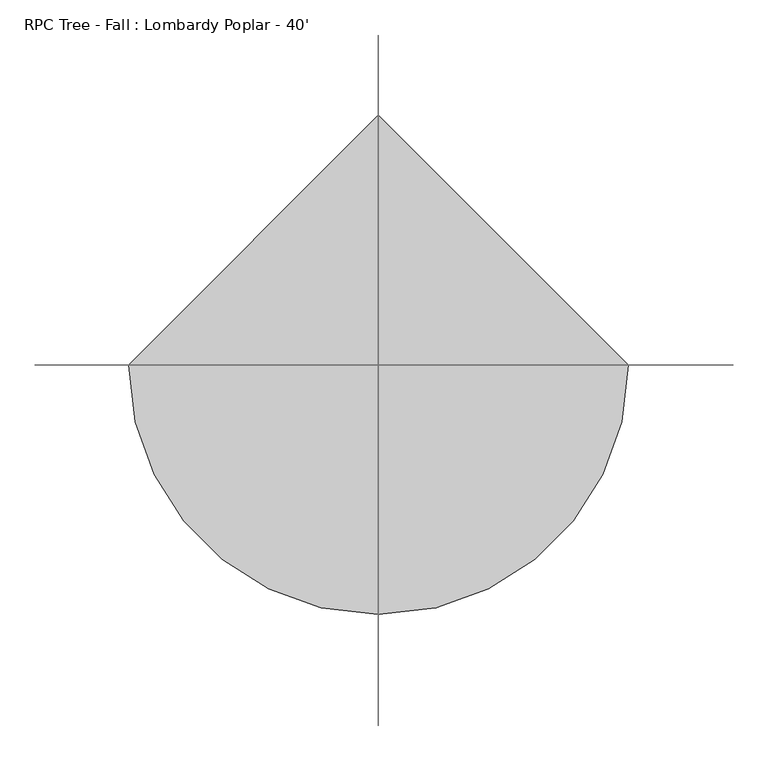
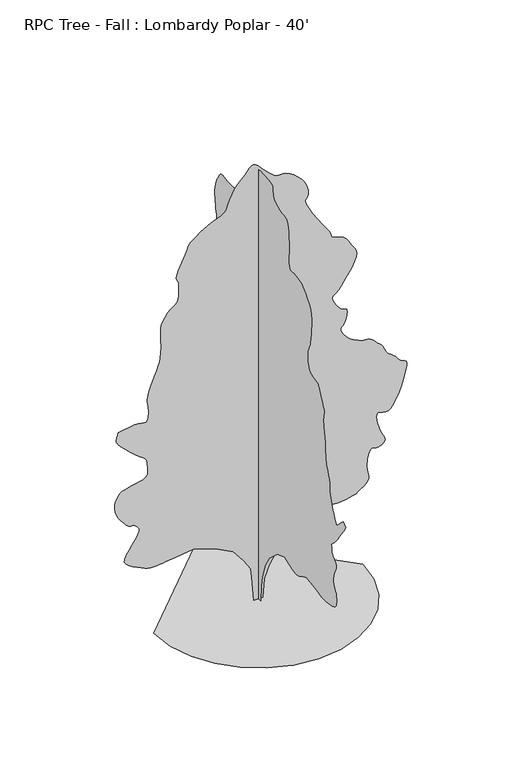
"""IFC4 building model written with IfcOpenShell, lengths in millimetres: geographic element geometry, RPC Tree - Fall : Lombardy Poplar - 40'."""

from ifc_helpers import new_model, si_unit, origin, place, context, project, spatial, triangles, source, transform, mapped, element, save


def rpc_tree_fall_lombardy_poplar_40_01077960(model_context):
    return source(origin(), model_context, "Body", "Tessellation", [
        triangles([(0.0009695, 113.8156909, 0.0), (0.0009695, -104.8345258, 0.0), (0.0009695, -123.055434, 437.3009239), (0.0009695, -177.7179314, 728.8340738), (0.0009695, -323.483707, 1129.6911467), (0.0009695, -505.6928613, 1439.4461494), (0.0009695, -870.1086628, 1767.420607), (0.0009695, -1216.3049732, 1894.9664555), (0.0009695, -1398.5142002, 1822.0838402), (0.0009695, -1476.390406, 1795.1523445), (0.0009695, -1552.9941605, 1770.6083485), (0.0009695, -1627.0451637, 1750.8472), (0.0009695, -1697.2735806, 1738.2588696), (0.0009695, -1762.3991112, 1735.2286766), (0.0009695, -1821.1516296, 1744.1542946), (0.0009695, -1872.2563591, 1767.420607), (0.0009695, -1919.1091679, 1797.0624023), (0.0009695, -1965.9644474, 1823.8364948), (0.0009695, -2012.8172562, 1848.2204716), (0.0009695, -2059.6700649, 1870.6891582), (0.0009695, -2106.5227283, 1891.7279903), (0.0009695, -2153.3780079, 1911.8067066), (0.0009695, -2200.2308167, 1931.4103065), (0.0009695, -2582.8711235, 1876.7470734), (0.0009695, -2649.2156204, 1861.2353748), (0.0009695, -2715.4080917, 1846.3611374), (0.0009695, -2781.27006, 1832.7619675), (0.0009695, -2846.6750793, 1821.0754715), (0.0009695, -2911.4196739, 1811.9366398), (0.0009695, -2975.3765259, 1805.987875), (0.0009695, -3038.3939003, 1803.8619873), (0.0009695, -3111.6472778, 1806.252103), (0.0009695, -3200.5217949, 1814.0625275), (0.0009695, -3296.0764275, 1828.2459641), (0.0009695, -3389.4213112, 1849.7596218), (0.0009695, -3471.5901329, 1879.5614365), (0.0009695, -3533.6930283, 1918.6062916), (0.0009695, -3566.7892639, 1967.8516869), (0.0009695, -3579.2353065, 2021.4507408), (0.0009695, -3585.9154221, 2073.1371208), (0.0009695, -3587.8205383, 2123.2333363), (0.0009695, -3585.9154221, 2172.0521587), (0.0009695, -3581.1401321, 2219.915807), (0.0009695, -3574.4347275, 2267.139378), (0.0009695, -3566.7892639, 2314.0455265), (0.0009695, -3532.0422569, 2353.5170998), (0.0009695, -3499.7078934, 2395.5361919), (0.0009695, -3472.1235306, 2442.6555542), (0.0009695, -3451.7273918, 2497.4231415), (0.0009695, -3440.907122, 2562.3988266), (0.0009695, -3441.9992065, 2640.0972816), (0.0009695, -3457.4677391, 2733.1372421), (0.0009695, -3484.5187042, 2825.1865654), (0.0009695, -3515.3799019, 2900.6752716), (0.0009695, -3544.9708282, 2963.0830902), (0.0009695, -3568.1862717, 3015.940329), (0.0009695, -3579.9210205, 3062.7525879), (0.0009695, -3575.0695724, 3106.9993057), (0.0009695, -3548.5775848, 3152.2110809), (0.0009695, -3509.7918709, 3193.1050964), (0.0009695, -3472.6063499, 3225.0836678), (0.0009695, -3438.6212151, 3252.6171616), (0.0009695, -3409.3857903, 3280.1253662), (0.0009695, -3386.5511375, 3312.1039375), (0.0009695, -3371.6668716, 3352.997953), (0.0009695, -3366.3581841, 3407.3030685), (0.0009695, -3362.7005585, 3460.5158089), (0.0009695, -3354.9027786, 3498.4634926), (0.0009695, -3347.7145546, 3525.8699593), (0.0009695, -3345.9620453, 3547.5360786), (0.0009695, -3354.4202499, 3568.2624298), (0.0009695, -3377.8388786, 3592.7987228), (0.0009695, -3421.0188011, 3625.9458275), (0.0009695, -3481.5215034, 3679.8698616), (0.0009695, -3552.5654228, 3760.5655174), (0.0009695, -3632.3465996, 3863.5624283), (0.0009695, -3719.1381042, 3984.4155167), (0.0009695, -3811.2130074, 4118.6541252), (0.0009695, -3906.7676399, 4261.8084686), (0.0009695, -4004.1003616, 4409.432888), (0.0009695, -3894.7788368, 4518.779702), (0.0009695, -3749.0086647, 4391.221209), (0.0009695, -3603.2382019, 4227.2390671), (0.0009695, -3579.7434151, 4258.785688), (0.0009695, -3555.9689941, 4292.2630051), (0.0009695, -3531.5088593, 4329.5499733), (0.0009695, -3506.1342453, 4372.5775795), (0.0009695, -3479.4643616, 4423.2506493), (0.0009695, -3451.1939941, 4483.4992973), (0.0009695, -3421.0188011, 4555.2033508), (0.0009695, -3390.0055779, 4628.5837555), (0.0009695, -3360.2623352, 4695.8683113), (0.0009695, -3333.0587631, 4762.2383881), (0.0009695, -3309.6910034, 4832.7233299), (0.0009695, -3291.4028755, 4912.4536377), (0.0009695, -3279.5158104, 5006.5351044), (0.0009695, -3275.248629, 5120.0473618), (0.0009695, -3267.0697678, 5234.8554703), (0.0009695, -3245.5050957, 5333.3820145), (0.0009695, -3215.0252701, 5421.7481323), (0.0009695, -3180.0747871, 5505.9238083), (0.0009695, -3145.0993057, 5592.0551788), (0.0009695, -3114.6191895, 5686.1110657), (0.0009695, -3093.0545174, 5794.238768), (0.0009695, -3079.5672592, 5892.1298859), (0.0009695, -3069.8899429, 5959.4403122), (0.0009695, -3063.4130127, 6007.9286316), (0.0009695, -3059.4760437, 6049.4319122), (0.0009695, -3057.4691895, 6095.6854843), (0.0009695, -3056.7073174, 6158.5246719), (0.0009695, -3056.6055794, 6249.735965), (0.0009695, -3052.5671631, 6343.1320084), (0.0009695, -3042.1532639, 6412.2958099), (0.0009695, -3027.9291321, 6468.709227), (0.0009695, -3012.4097305, 6523.8523727), (0.0009695, -2998.1858894, 6589.2065231), (0.0009695, -2987.7716995, 6676.2017944), (0.0009695, -2983.7332832, 6796.3688782), (0.0009695, -2989.2957344, 6908.7381821), (0.0009695, -3001.5638809, 6976.78461), (0.0009695, -3013.8576073, 7018.6948425), (0.0009695, -3019.4200584, 7052.6288177), (0.0009695, -3011.6222786, 7096.7737976), (0.0009695, -2983.7332832, 7169.2908829), (0.0009695, -2929.0723755, 7288.340593), (0.0009695, -2866.7410057, 7418.1088348), (0.0009695, -2818.7857933, 7514.4256302), (0.0009695, -2782.7688057, 7582.8528488), (0.0009695, -2756.3021072, 7628.9541046), (0.0009695, -2737.0233421, 7658.3418457), (0.0009695, -2722.5201576, 7676.5535248), (0.0009695, -2710.4043274, 7689.2027527), (0.0009695, -2636.5666832, 7701.2421341), (0.0009695, -2564.8117607, 7715.3901077), (0.0009695, -2497.1818771, 7733.6523651), (0.0009695, -2435.7748695, 7758.1380798), (0.0009695, -2382.6507866, 7790.9296829), (0.0009695, -2339.8900246, 7834.0584457), (0.0009695, -2309.5548122, 7889.6335419), (0.0009695, -2289.3160767, 7951.0257248), (0.0009695, -2274.8152176, 8010.5377899), (0.0009695, -2265.0921192, 8068.4243729), (0.0009695, -2259.1968395, 8125.0662643), (0.0009695, -2256.1691174, 8180.7425171), (0.0009695, -2255.0515984, 8235.7589264), (0.0009695, -2254.8940498, 8290.4707031), (0.0009695, -2285.970932, 8345.7405853), (0.0009695, -2316.0901691, 8404.491069), (0.0009695, -2344.2968777, 8470.25159), (0.0009695, -2369.6358833, 8546.5277481), (0.0009695, -2391.1521572, 8636.8495605), (0.0009695, -2407.8857288, 8744.6726303), (0.0009695, -2418.8812786, 8873.551973), (0.0009695, -2430.0903328, 9004.9206985), (0.0009695, -2443.8493767, 9121.3031296), (0.0009695, -2453.7833633, 9227.8303482), (0.0009695, -2453.5168098, 9329.5572784), (0.0009695, -2436.6765587, 9431.5888412), (0.0009695, -2396.8874176, 9539.0561188), (0.0009695, -2327.7766651, 9657.0390335), (0.0009695, -2247.8811058, 9768.2398041), (0.0009695, -2177.228587, 9854.8798645), (0.0009695, -2111.6764835, 9921.4269653), (0.0009695, -2047.0792637, 9972.3796692), (0.0009695, -1979.2969185, 10012.156311), (0.0009695, -1904.1815907, 10045.2519653), (0.0009695, -1817.5931259, 10076.1128723), (0.0009695, -1725.5334835, 10094.8326599), (0.0009695, -1638.891679, 10096.3058258), (0.0009695, -1560.8554539, 10092.3688568), (0.0009695, -1494.6124043, 10094.8326599), (0.0009695, -1443.3501263, 10115.4325653), (0.0009695, -1410.2540359, 10166.0038971), (0.0009695, -1398.5142002, 10258.3319824), (0.0009695, -1400.4267288, 10362.6756134), (0.0009695, -1404.8895378, 10448.1971375), (0.0009695, -1409.9898079, 10525.1087219), (0.0009695, -1413.8125397, 10603.619046), (0.0009695, -1414.4501461, 10693.9414398), (0.0009695, -1409.9898079, 10806.2345856), (0.0009695, -1398.5142002, 10950.7350677), (0.0009695, -1382.6849339, 11097.4458801), (0.0009695, -1365.5779839, 11211.9737732), (0.0009695, -1345.9235149, 11297.8255096), (0.0009695, -1322.4438435, 11358.4811096), (0.0009695, -1293.8637566, 11397.4694275), (0.0009695, -1258.9083321, 11418.297226), (0.0009695, -1216.3049732, 11424.470105), (0.0009695, -1155.4822323, 11429.9813965), (0.0009695, -1073.3006933, 11446.3641174), (0.0009695, -979.6484882, 11473.2380585), (0.0009695, -884.3986336, 11510.3218414), (0.0009695, -797.4393339, 11557.2608368), (0.0009695, -728.6460766, 11613.8015717), (0.0009695, -687.9020519, 11679.5615112), (0.0009695, -672.8677952, 11749.3607391), (0.0009695, -668.0341513, 11816.289212), (0.0009695, -663.5180752, 11877.4785004), (0.0009695, -649.4413908, 11930.0811035), (0.0009695, -615.9210531, 11971.2041748), (0.0009695, -553.0790314, 11997.9757965), (0.0009695, -451.0296281, 12007.5263763), (0.0009695, -327.7864603, 12011.2087097), (0.0009695, -210.2816959, 12019.0070709), (0.0009695, -102.0189364, 12026.1694244), (0.0009695, -6.5056406, 12027.9216431), (0.0009695, 72.7523407, 12019.4895996), (0.0009695, 132.2489498, 11996.0700989), (0.0009695, 168.4781792, 11952.8657593), (0.0009695, 190.2581361, 11903.7920105), (0.0009695, 211.0820467, 11861.400412), (0.0009695, 234.4553475, 11819.0076508), (0.0009695, 263.8852554, 11769.9094849), (0.0009695, 302.8767344, 11707.4505066), (0.0009695, 354.9364746, 11624.9008942), (0.0009695, 423.5697126, 11515.57966), (0.0009695, 499.5867296, 11399.1204895), (0.0009695, 572.09851, 11297.9778259), (0.0009695, 642.0601553, 11209.5867096), (0.0009695, 710.4292379, 11131.3798553), (0.0009695, 778.1582434, 11060.8446259), (0.0009695, 846.2072874, 10995.3881561), (0.0009695, 915.531399, 10932.4978088), (0.0009695, 983.7404623, 10880.5556305), (0.0009695, 1048.444289, 10847.0786041), (0.0009695, 1110.5954372, 10828.282077), (0.0009695, 1171.1565662, 10820.3069824), (0.0009695, 1231.077618, 10819.3407623), (0.0009695, 1291.3160923, 10821.5766724), (0.0009695, 1352.8322502, 10823.1765747), (0.0009695, 1419.1287849, 10828.7646057), (0.0009695, 1490.5254444, 10841.0324615), (0.0009695, 1563.194846, 10853.3014801), (0.0009695, 1633.3164379, 10858.8639313), (0.0009695, 1697.0626923, 10851.0655701), (0.0009695, 1750.6084064, 10823.1765747), (0.0009695, 1790.1333195, 10768.5159576), (0.0009695, 1824.1844387, 10700.9526398), (0.0009695, 1861.7408672, 10636.2333344), (0.0009695, 1899.617189, 10570.5745514), (0.0009695, 1934.6234825, 10500.1404785), (0.0009695, 1963.5743317, 10421.0953033), (0.0009695, 1983.2847565, 10329.6299561), (0.0009695, 1990.5617832, 10221.8830444), (0.0009695, 1988.4357502, 10111.0130676), (0.0009695, 1982.4871307, 10010.9877777), (0.0009695, 1973.3507698, 9919.2433777), (0.0009695, 1961.6642738, 9833.2381622), (0.0009695, 1948.0651039, 9750.4350769), (0.0009695, 1933.1908665, 9668.2656738), (0.0009695, 1917.6791679, 9584.1667374), (0.0009695, 1914.3314072, 9505.3761978), (0.0009695, 1931.0649788, 9438.0663528), (0.0009695, 1961.1842159, 9378.0967575), (0.0009695, 1997.9989746, 9321.3025497), (0.0009695, 2034.813588, 9263.5682831), (0.0009695, 2064.9328251, 9200.7290955), (0.0009695, 2081.6663967, 9128.6439606), (0.0009695, 2081.1888096, 9058.6668365), (0.0009695, 2066.6854797, 9001.7964706), (0.0009695, 2041.9840805, 8953.1808334), (0.0009695, 2010.9071983, 8908.0707962), (0.0009695, 1977.2826519, 8861.6904877), (0.0009695, 1944.9307022, 8809.2646179), (0.0009695, 1917.6791679, 8745.9934799), (0.0009695, 1901.8472855, 8673.7048691), (0.0009695, 1900.361475, 8598.2164536), (0.0009695, 1911.9412914, 8520.8229218), (0.0009695, 1935.3142834, 8442.7939636), (0.0009695, 1969.2055286, 8365.374852), (0.0009695, 2012.3422852, 8289.8864365), (0.0009695, 2063.4443985, 8217.5978256), (0.0009695, 2116.1951031, 8158.060762), (0.0009695, 2166.3955273, 8113.7884644), (0.0009695, 2215.9584904, 8075.6123062), (0.0009695, 2266.796521, 8034.2101822), (0.0009695, 2320.8222931, 7980.4134659), (0.0009695, 2379.9457191, 7904.924469), (0.0009695, 2446.0820892, 7798.5239868), (0.0009695, 2515.4595406, 7684.1478287), (0.0009695, 2583.8870499, 7588.5931961), (0.0009695, 2652.6194824, 7508.3039108), (0.0009695, 2722.9518173, 7439.8511124), (0.0009695, 2796.1546165, 7379.653624), (0.0009695, 2873.4972794, 7324.2558426), (0.0009695, 2956.2759476, 7270.103334), (0.0009695, 3039.9940933, 7227.3042023), (0.0009695, 3119.5720848, 7202.0063278), (0.0009695, 3195.3148453, 7185.0137604), (0.0009695, 3267.5522964, 7167.0555542), (0.0009695, 3336.6149414, 7138.9125046), (0.0009695, 3402.807122, 7091.3130844), (0.0009695, 3466.4593414, 7015.0113464), (0.0009695, 3525.2604034, 6921.5903046), (0.0009695, 3575.4506538, 6829.7441666), (0.0009695, 3615.1508469, 6741.0728348), (0.0009695, 3642.3797081, 6657.2023727), (0.0009695, 3655.3082794, 6579.6815231), (0.0009695, 3651.9552864, 6510.1619293), (0.0009695, 3630.4414833, 6450.1673355), (0.0009695, 3590.004998, 6392.5348068), (0.0009695, 3534.6075073, 6330.4316208), (0.0009695, 3469.3295151, 6266.1192673), (0.0009695, 3399.2512344, 6201.7813339), (0.0009695, 3329.5028755, 6139.6781479), (0.0009695, 3265.1646515, 6082.0456192), (0.0009695, 3211.3676445, 6031.0934967), (0.0009695, 3161.7869499, 5985.0939789), (0.0009695, 3109.3613708, 5939.7298874), (0.0009695, 3057.8758507, 5893.4001572), (0.0009695, 3011.1906189, 5844.5304657), (0.0009695, 2973.1159081, 5791.5209106), (0.0009695, 2947.4366615, 5732.7710083), (0.0009695, 2938.0386887, 5666.680275), (0.0009695, 2934.1778778, 5597.4141541), (0.0009695, 2924.8816429, 5529.7235184), (0.0009695, 2913.6547119, 5463.0235199), (0.0009695, 2904.0535538, 5396.6025742), (0.0009695, 2899.5323181, 5329.8764145), (0.0009695, 2903.6218941, 5262.2113586), (0.0009695, 2919.8270096, 5192.9452377), (0.0009695, 2944.8458313, 5126.3719757), (0.0009695, 2972.7351173, 5066.5046997), (0.0009695, 3003.0117577, 5012.2248734), (0.0009695, 3035.1935143, 4962.3901245), (0.0009695, 3068.8231476, 4915.908078), (0.0009695, 3103.4178383, 4871.6613602), (0.0009695, 3138.4697685, 4828.5323067), (0.0009695, 3181.1415825, 4835.3141602), (0.0009695, 3222.035598, 4836.0760323), (0.0009695, 3259.4243042, 4824.696785), (0.0009695, 3291.5807716, 4795.1567276), (0.0009695, 3316.7013313, 4741.4102989), (0.0009695, 3333.0587631, 4657.3619408), (0.0009695, 3338.9008484, 4536.9916718), (0.0009695, 3338.9008484, 3935.6984322), (0.0009695, 3345.6065437, 3757.6444748), (0.0009695, 3361.2273926, 3611.1377197), (0.0009695, 3379.0582809, 3492.0371407), (0.0009695, 3392.4440918, 3396.2031647), (0.0009695, 3394.6791298, 3319.4953468), (0.0009695, 3379.0582809, 3257.747953), (0.0009695, 3338.9008484, 3206.8719887), (0.0009695, 3281.573243, 3178.2461197), (0.0009695, 3221.7053856, 3174.1568344), (0.0009695, 3163.4380119, 3176.747374), (0.0009695, 3110.9106949, 3168.187722), (0.0009695, 3068.2388809, 3130.6466995), (0.0009695, 3039.6130119, 3046.21726), (0.0009695, 3029.1482437, 2897.119384), (0.0009695, 3036.0571243, 2732.8070297), (0.0009695, 3053.1514297, 2608.9823204), (0.0009695, 3075.0460236, 2517.0268867), (0.0009695, 3096.3057724, 2448.3400909), (0.0009695, 3111.4949615, 2394.3144642), (0.0009695, 3115.2034561, 2346.3441364), (0.0009695, 3102.0208305, 2295.8261444), (0.0009695, 3089.0669701, 2254.1778145), (0.0009695, 3089.803553, 2232.6106716), (0.0009695, 3093.4355988, 2222.1992432), (0.0009695, 3089.0669701, 2214.0179111), (0.0009695, 3065.9021049, 2199.1436737), (0.0009695, 3013.0954445, 2168.6510582), (0.0009695, 2919.8270096, 2113.6169174), (0.0009695, 2822.3419716, 2052.8450455), (0.0009695, 2753.55867, 2008.9666191), (0.0009695, 2697.5010452, 1978.7940422), (0.0009695, 2638.2683235, 1959.1395733), (0.0009695, 2559.9350235, 1946.8154709), (0.0009695, 2446.5088074, 1938.6341389), (0.0009695, 2282.0948605, 1931.4103065), (0.0009695, 2105.8903542, 1933.6938881), (0.0009695, 1963.4702682, 1951.9132702), (0.0009695, 1848.4591198, 1979.6982021), (0.0009695, 1754.4869488, 2010.665934), (0.0009695, 1675.1755108, 2038.4483952), (0.0009695, 1604.1522297, 2056.670248), (0.0009695, 1535.0414772, 2058.9536842), (0.0009695, 1460.510416, 2049.0198429), (0.0009695, 1378.3312752, 2035.2631245), (0.0009695, 1289.7769421, 2018.3163391), (0.0009695, 1196.1221935, 1998.8218895), (0.0009695, 1098.6447859, 1977.4122952), (0.0009695, 998.6146271, 1954.7301041), (0.0009695, 897.3120169, 1931.4103065), (0.0009695, 532.8936719, 1639.8747585), (0.0009695, 314.2457534, 1166.1349977), (0.0009695, 168.4781792, 601.2881527), (120.1776209, 0.0005334, 0.0085345), (-116.69275, 0.0005334, 0.0085345), (-171.3552383, 0.0004849, 655.9590162), (-207.7973272, 0.0004849, 911.0508585), (-390.006209, 0.0004607, 1202.5839357), (-663.3174334, 0.0004364, 1548.7803188), (-1137.0596649, 0.0004122, 1803.8721611), (-1720.1284355, 0.0004122, 1986.078772), (-2193.8681236, 0.0004122, 1931.4180096), (-2467.1819641, 0.0004122, 1894.9766293), (-2533.7959213, 0.0004122, 1885.46689), (-2607.4327057, 0.0004122, 1874.6820831), (-2686.1473778, 0.0004122, 1865.812421), (-2768.0621452, 0.0004122, 1862.0405582), (-2851.2468933, 0.0004122, 1866.556707), (-2933.7967964, 0.0004122, 1882.5459927), (-3013.8067383, 0.0004122, 1913.1960114), (-3104.2814484, 0.0004122, 1955.5886272), (-3210.9865631, 0.0004122, 2004.6715324), (-3321.222567, 0.0004122, 2060.4522846), (-3422.2126236, 0.0004122, 2122.9234715), (-3501.2066391, 0.0003879, 2192.0875637), (-3545.4533569, 0.0003879, 2267.9445614), (-3542.2021019, 0.0003879, 2350.4969353), (-3495.1869484, 0.0003879, 2447.2326004), (-3424.930481, 0.0003879, 2559.9094437), (-3343.8031654, 0.0003637, 2679.898922), (-3264.2757523, 0.0003637, 2798.6437088), (-3198.7692856, 0.0003637, 2907.4824142), (-3159.7295174, 0.0003394, 2997.8300972), (-3159.5772011, 0.0003394, 3061.1015259), (-3182.9958298, 0.0003394, 3103.1893639), (-3206.4147491, 0.0003394, 3136.6411011), (-3229.8589577, 0.0003394, 3162.9554832), (-3253.2775864, 0.0003394, 3183.5039383), (-3276.6962151, 0.0003394, 3199.7599228), (-3300.1404236, 0.0003394, 3213.1457336), (-3323.559343, 0.0003394, 3225.1089569), (-3347.1558678, 0.0003394, 3221.5783585), (-3371.6921608, 0.0003394, 3220.486274), (-3398.1335701, 0.0003394, 3224.1438995), (-3427.4704422, 0.0003394, 3234.9897491), (-3460.6175468, 0.0003394, 3255.3858879), (-3498.5396507, 0.0003394, 3287.7199608), (-3542.2021019, 0.0003394, 3334.4304817), (-3593.6370438, 0.0003394, 3395.5174507), (-3650.1519081, 0.0003152, 3468.3897469), (-3705.7270042, 0.0003152, 3551.4730476), (-3754.2664833, 0.0003152, 3643.1668694), (-3789.7500732, 0.0003152, 3741.8713097), (-3806.1330849, 0.0002909, 3845.9855942), (-3797.2937988, 0.0002909, 3953.9354004), (-3771.4366562, 0.0002909, 4051.5730453), (-3739.8138771, 0.0002909, 4128.1791252), (-3701.2057686, 0.0002909, 4187.2342415), (-3654.2920624, 0.0002667, 4232.2937004), (-3597.828067, 0.0002667, 4266.812233), (-3530.518222, 0.0002667, 4294.3457268), (-3451.117836, 0.0002667, 4318.3486221), (-3356.8078949, 0.0002667, 4338.3131012), (-3252.3378181, 0.0002667, 4355.4326958), (-3147.5122398, 0.0002667, 4375.7270966), (-3052.2622398, 0.0002667, 4405.2674446), (-2976.4689011, 0.0002667, 4450.0981384), (-2929.9868546, 0.0002667, 4516.2906097), (-2922.6971832, 0.0002667, 4609.8895477), (-2933.5936111, 0.0002425, 4707.6283493), (-2938.4197701, 0.0002425, 4784.9713028), (-2942.3058701, 0.0002425, 4846.0582718), (-2950.332415, 0.0002425, 4895.0291199), (-2967.578746, 0.0002425, 4936.0504532), (-2999.2018158, 0.0002425, 4973.2359741), (-3050.2556763, 0.0002425, 5010.7517075), (-3135.4978569, 0.0002182, 5072.041571), (-3254.8777794, 0.0002182, 5168.7141586), (-3391.1232422, 0.0002182, 5287.0778641), (-3527.0637817, 0.0002182, 5413.3916656), (-3645.4783562, 0.000194, 5533.9906998), (-3729.1459236, 0.000194, 5635.1333633), (-3760.8704407, 0.000194, 5703.129213), (-3759.2702477, 0.000194, 5747.3247711), (-3754.799881, 0.000194, 5786.7456207), (-3747.9418694, 0.000194, 5822.178923), (-3739.1787415, 0.0001697, 5854.4112579), (-3728.9933167, 0.0001697, 5884.2815277), (-3717.8428345, 0.0001697, 5912.5263153), (-3706.2095329, 0.0001697, 5940.0089401), (-3268.8984352, 0.0001697, 6012.8818176), (-3174.1312546, 0.0001697, 6014.48172), (-3093.0545174, 0.0001697, 5998.8605804), (-3026.0240158, 0.0001697, 5982.2743835), (-2973.319384, 0.0001697, 5981.0046936), (-2935.2955421, 0.0001697, 6011.2813339), (-2912.232415, 0.0001697, 6089.3864502), (-2904.4852135, 0.0001697, 6231.5242859), (-2910.9624344, 0.0001455, 6377.1421417), (-2925.0848282, 0.0001455, 6470.4870255), (-2938.9022987, 0.0001455, 6535.1301727), (-2944.4394608, 0.0001455, 6594.6678177), (-2933.6953491, 0.0001212, 6672.7217743), (-2898.7448662, 0.0001212, 6792.8126999), (-2831.5873375, 0.0001212, 6978.5879883), (-2754.346122, 9.7e-05, 7175.5649185), (-2693.3861801, 9.7e-05, 7325.0435852), (-2647.0567406, 9.7e-05, 7444.2456116), (-2613.8081886, 7.27e-05, 7550.3920395), (-2592.0150421, 7.27e-05, 7660.678331), (-2580.127977, 7.27e-05, 7792.3011108), (-2576.4956406, 4.85e-05, 7962.5064194), (-2580.0009499, 4.85e-05, 8135.9626923), (-2586.7063545, 4.85e-05, 8272.4363388), (-2590.8467995, 2.42e-05, 8381.8087326), (-2586.7063545, 2.42e-05, 8473.985083), (-2568.5455444, 2.42e-05, 8558.8211838), (-2530.6106506, 2.42e-05, 8646.1972458), (-2467.1819641, 0.0, 8746.0190598), (-2393.5550629, 0.0, 8838.8046753), (-2328.8511635, 0.0, 8903.8797729), (-2273.0728821, 0.0, 8949.1932861), (-2226.2200733, 0.0, 8982.7208908), (-2188.2902664, 0.0, 9012.4138458), (-2159.2860775, 0.0, 9046.2460831), (-2139.2048904, 0.0, 9092.1950226), (-2125.7124001, -2.42e-05, 9135.3493652), (-2116.0452576, -2.42e-05, 9162.8575699), (-2109.5630951, -2.42e-05, 9185.920697), (-2105.6338291, -2.42e-05, 9215.6642303), (-2103.6144756, -2.42e-05, 9263.2636505), (-2102.8701897, -2.42e-05, 9339.8700211), (-2102.7661263, -2.42e-05, 9456.6332428), (-2113.0708752, -4.85e-05, 9567.5549606), (-2136.1264446, -4.85e-05, 9634.4840149), (-2160.137043, -4.85e-05, 9680.3817947), (-2173.3094948, -4.85e-05, 9728.1846909), (-2163.855566, -4.85e-05, 9800.8540924), (-2119.9745235, -7.27e-05, 9921.3258087), (-2029.8808949, -7.27e-05, 10112.5618103), (-1939.4672276, -7.27e-05, 10305.830246), (-1888.8958958, -9.7e-05, 10431.5097839), (-1857.7656738, -9.7e-05, 10511.3165405), (-1825.6805683, -9.7e-05, 10566.8654755), (-1772.2389175, -9.7e-05, 10619.9006104), (-1677.0450188, -9.7e-05, 10692.0369049), (-1519.6973557, -0.0001212, 10804.9648956), (-1341.6868549, -0.0001212, 10917.309201), (-1195.5481733, -0.0001212, 10985.3806274), (-1077.4586517, -0.0001212, 11027.29086), (-983.5905441, -0.0001212, 11061.2248352), (-910.1237349, -0.0001212, 11105.3698151), (-853.2303326, -0.0001455, 11177.8874817), (-809.0852074, -0.0001455, 11296.9371918), (-759.9464916, -0.0001455, 11440.4714539), (-694.8717573, -0.0001697, 11572.8563965), (-620.2365601, -0.0001697, 11691.8293671), (-542.413585, -0.0001697, 11795.2079407), (-467.775808, -0.0001697, 11880.7294647), (-402.7036534, -0.0001697, 11946.1847717), (-353.5649014, -0.000194, 11989.3146973), (-315.2642959, -0.000194, 12029.8529205), (-276.9611651, -0.000194, 12081.541626), (-236.4299363, -0.000194, 12133.2303314), (-191.4351718, -0.000194, 12173.7685547), (-139.7475292, -0.000194, 12191.9802338), (-79.1353495, -0.000194, 12176.7404663), (-7.3676139, -0.000194, 12116.8731903), (68.4904824, -0.000194, 12035.3130524), (139.8862108, -0.000194, 11962.0605469), (206.8199341, -0.0001697, 11896.4517609), (269.290376, -0.0001697, 11837.8797546), (327.3013518, -0.0001697, 11785.6573608), (380.8469934, -0.0001697, 11739.1753143), (429.9324057, -0.0001697, 11697.7987701), (477.3160323, -0.0001697, 11672.4491547), (527.8899076, -0.0001697, 11666.8622864), (584.8366133, -0.0001697, 11669.5795624), (651.343891, -0.0001697, 11669.0970337), (730.6019165, -0.0001697, 11653.9584229), (825.7958879, -0.0001697, 11612.684198), (940.1160175, -0.0001455, 11533.7913391), (1053.1051964, -0.0001455, 11434.3508972), (1143.4680674, -0.0001455, 11338.4148926), (1213.1096741, -0.0001455, 11245.0194305), (1263.9477047, -0.0001455, 11153.2238708), (1297.8921444, -0.0001212, 11062.0631561), (1316.8558125, -0.0001212, 10970.5978088), (1322.7537083, -0.0001212, 10877.8371918), (1310.6404942, -0.0001212, 10807.3019623), (1283.8688725, -0.0001212, 10768.6426941), (1256.7747414, -0.0001212, 10740.1444336), (1243.7064983, -9.7e-05, 10700.2154755), (1259.0074539, -9.7e-05, 10627.1141235), (1317.0158318, -9.7e-05, 10499.1998383), (1432.0777039, -7.27e-05, 10294.7809204), (1568.3356659, -7.27e-05, 10074.4362305), (1681.0074223, -4.85e-05, 9906.365094), (1771.0503273, -4.85e-05, 9780.3565063), (1839.4167938, -4.85e-05, 9686.22388), (1887.067083, -4.85e-05, 9613.757373), (1914.9562237, -4.85e-05, 9552.772142), (1924.041861, -2.42e-05, 9493.0571823), (1943.5896503, -2.42e-05, 9444.2892288), (1995.6494087, -2.42e-05, 9415.2822784), (2070.3380184, -2.42e-05, 9394.5812164), (2157.7773033, -2.42e-05, 9370.6797684), (2248.0842911, -2.42e-05, 9332.0972397), (2331.3809509, -2.42e-05, 9267.4035141), (2397.7841652, -2.42e-05, 9165.0928986), (2454.6240097, 0.0, 9055.2379761), (2511.1467224, 0.0, 8968.9542892), (2560.341394, 0.0, 8896.3866257), (2595.190139, 0.0, 8827.6541931), (2608.6773972, 0.0, 8752.8512009), (2593.7931313, 2.42e-05, 8662.1230179), (2543.5520119, 2.42e-05, 8545.5876892), (2481.3447624, 2.42e-05, 8432.1260101), (2431.8886242, 2.42e-05, 8349.5508179), (2390.080275, 2.42e-05, 8286.457576), (2350.8220608, 4.85e-05, 8231.3138489), (2309.0163277, 4.85e-05, 8172.6656845), (2259.5600441, 4.85e-05, 8099.0312256), (2197.3530853, 4.85e-05, 7998.9553574), (2127.0206051, 4.85e-05, 7904.0355698), (2060.8307499, 7.27e-05, 7844.1677124), (2005.159148, 7.27e-05, 7805.3311295), (1966.378521, 7.27e-05, 7773.5051651), (1950.8666771, 7.27e-05, 7734.6685822), (1964.9992447, 7.27e-05, 7674.8007248), (2015.1464745, 7.27e-05, 7579.8815186), (2080.6452381, 7.27e-05, 7478.1545883), (2137.5387131, 9.7e-05, 7404.1387573), (2187.2590794, 9.7e-05, 7353.262793), (2231.2468014, 9.7e-05, 7320.852562), (2270.9265015, 9.7e-05, 7302.3106705), (2307.7412601, 9.7e-05, 7293.0141449), (2343.1207867, 9.7e-05, 7288.340593), (2346.839455, 9.7e-05, 7260.6544922), (2349.4429298, 9.7e-05, 7230.9109589), (2349.8136921, 9.7e-05, 7197.027562), (2346.839455, 9.7e-05, 7156.9212891), (2339.4022636, 9.7e-05, 7108.5341263), (2326.3873604, 0.0001212, 7049.7842239), (2306.6795517, 0.0001212, 6978.5879883), (2277.832766, 0.0001212, 6914.427951), (2243.2507198, 0.0001212, 6871.273027), (2210.5813477, 0.0001212, 6838.9901138), (2187.4724384, 0.0001212, 6807.3158844), (2181.5771587, 0.0001212, 6766.0922379), (2200.5406815, 0.0001212, 6705.1064255), (2252.0163185, 0.0001455, 6614.1747665), (2322.1379105, 0.0001455, 6519.5090332), (2391.3020027, 0.0001455, 6450.3452316), (2458.553421, 0.0001455, 6400.9424332), (2522.9372818, 0.0001455, 6365.5602905), (2583.5059685, 0.0001455, 6338.4584564), (2639.2842499, 0.0001455, 6313.9221634), (2689.322184, 0.0001455, 6286.184903), (2738.2427444, 0.0001455, 6263.7822006), (2790.6680328, 0.0001455, 6254.1048843), (2845.659153, 0.0001697, 6249.8632828), (2902.2248863, 0.0001697, 6243.6909851), (2959.4507538, 0.0001697, 6228.2989014), (3016.3466995, 0.0001697, 6196.3200394), (3071.9473755, 0.0001697, 6140.4403107), (3121.4519119, 0.0001697, 6084.0774719), (3162.3712166, 0.0001697, 6048.746489), (3197.2199615, 0.0001697, 6024.2607742), (3228.5633972, 0.0001697, 6000.4104858), (3258.9417755, 0.0001697, 5966.9840378), (3290.9203468, 0.0001697, 5913.8215851), (3327.0390724, 0.000194, 5830.687706), (3367.3235321, 0.000194, 5746.3091354), (3410.4525856, 0.000194, 5689.0573975), (3457.0869484, 0.000194, 5648.0366455), (3507.8614655, 0.000194, 5612.4510269), (3563.4365616, 0.000194, 5571.430275), (3624.4217926, 0.000194, 5514.178537), (3691.4522942, 0.0002182, 5429.8255463), (3759.9306725, 0.0002182, 5354.920816), (3822.0335678, 0.0002182, 5319.208461), (3873.620826, 0.0002182, 5301.6827866), (3910.5270035, 0.0002182, 5281.2863571), (3928.6625244, 0.0002182, 5236.989061), (3923.8110764, 0.0002182, 5147.7334625), (3891.883374, 0.0002425, 4992.5144485), (3839.8897453, 0.0002425, 4801.4304726), (3779.2600159, 0.0002667, 4621.8274818), (3712.6105957, 0.0002667, 4458.4801849), (3642.4302864, 0.0002667, 4316.1641624), (3571.3104996, 0.0002909, 4199.6799934), (3501.7653259, 0.0002909, 4113.777388), (3436.3605972, 0.0002909, 4063.2569252), (3368.5935127, 0.0002909, 4052.055574), (3295.6956367, 0.0002909, 4067.2956322), (3225.9981468, 0.0002909, 4088.6059593), (3167.7813515, 0.0002909, 4095.5657089), (3129.3258499, 0.0002909, 4067.7781609), (3118.9119507, 0.0002909, 3984.8471764), (3144.8452515, 0.0002909, 3826.3769073), (3196.8388802, 0.0003152, 3648.5264259), (3252.998243, 0.0003152, 3514.6686081), (3304.0521034, 0.0003152, 3415.2278755), (3340.7550957, 0.0003394, 3340.6280685), (3353.8615631, 0.0003394, 3281.3444778), (3334.1764275, 0.0003394, 3227.8015251), (3272.3784554, 0.0003394, 3170.4230507), (3191.911274, 0.0003394, 3134.2534561), (3121.6295174, 0.0003394, 3135.3711205), (3060.5934174, 0.0003394, 3150.839653), (3007.8379166, 0.0003394, 3157.6976646), (2962.4226654, 0.0003394, 3132.9834755), (2923.3828972, 0.0003394, 3053.7862747), (2889.7532639, 0.0003637, 2897.119384), (2876.0881096, 0.0003637, 2719.1165863), (2887.6196732, 0.0003879, 2584.1155243), (2909.3366615, 0.0003879, 2481.6546272), (2926.3039398, 0.0003879, 2401.1749466), (2923.4846352, 0.0003879, 2332.1708736), (2885.9180328, 0.0003879, 2264.1218296), (2798.6437088, 0.0003879, 2186.5098518), (2701.5906212, 0.0004122, 2115.113047), (2635.7792313, 0.0004122, 2068.2602383), (2587.7987297, 0.0004122, 2039.2560493), (2544.2885948, 0.0004122, 2021.4075748), (2491.8603996, 0.0004122, 2008.0191479), (2417.1185955, 0.0004122, 1992.4007698), (2306.6795517, 0.0004122, 1967.8592445), (2182.1079403, 0.0004122, 1946.8763683), (2070.9247559, 0.0004122, 1942.7844669), (1968.6644279, 0.0004122, 1950.1707893), (1870.8670544, 0.0004122, 1963.60994), (1773.0695354, 0.0004122, 1977.6865517), (1670.8093529, 0.0004122, 1986.9829319), (1559.6260231, 0.0004122, 1986.078772), (1454.709026, 0.0004122, 1976.1447853), (1371.7857445, 0.0004122, 1962.3882122), (1307.1885246, 0.0004122, 1945.4412815), (1257.2547993, 0.0004122, 1925.9468319), (1218.3166964, 0.0004122, 1904.5372375), (1186.70896, 0.0004122, 1881.8550465), (1158.7664795, 0.0004122, 1858.5353943), (1158.4464409, 0.0004364, 1761.2688023), (1156.2163445, 0.0004364, 1666.0722874), (1150.1584293, 0.0004364, 1575.0234844), (1138.3677246, 0.0004364, 1490.1876743), (1118.9240713, 0.0004364, 1413.6372597), (1089.9198824, 0.0004607, 1347.4475498), (1049.4399405, 0.0004607, 1293.6884766), (1004.179767, 0.0004607, 1251.6160446), (961.7897673, 0.0004607, 1218.1490467), (921.7874125, 0.0004607, 1191.8550121), (883.7001297, 0.0004607, 1171.2962379), (847.045463, 0.0004607, 1155.0403261), (811.3483686, 0.0004607, 1141.6519718), (776.1287888, 0.0004607, 1129.7013205), (466.3737496, 0.0004607, 1129.7013205), (284.1645772, 0.0004849, 856.3875526), (156.6199641, 0.0005092, 510.1912059), (-2766.0555817, 0.0, 0.0100862), (-2692.9292313, -633.8001217, 0.0100862), (-2484.680024, -1215.8427195, 0.0100862), (-2157.9602863, -1729.4553371, 0.0100862), (-1729.4553371, -2157.9602863, 0.0100862), (-1215.8427195, -2484.680024, 0.0100862), (-633.8001217, -2692.9292313, 0.0100862), (0.0001209, -2766.0555817, 0.0100862), (633.8001217, -2692.9292313, 0.0100862), (1215.8427195, -2484.680024, 0.0100862), (1729.4553371, -2157.9602863, 0.0100862), (2157.9602863, -1729.4553371, 0.0100862), (2484.680024, -1215.8427195, 0.0100862), (2692.9292313, -633.8001217, 0.0100862), (2766.0555817, 0.0002425, 0.0100862), (-0.0003627, 2766.0555817, 0.0100862)], [[1, 2, 3], [388, 1, 3], [388, 3, 4], [387, 388, 4], [387, 4, 5], [80, 81, 82], [79, 80, 82], [79, 82, 83], [78, 79, 83], [77, 78, 83], [387, 5, 6], [386, 387, 6], [76, 77, 83], [386, 6, 7], [359, 360, 361], [359, 361, 362], [385, 386, 7], [75, 76, 83], [75, 83, 84], [75, 84, 85], [74, 75, 85], [73, 74, 85], [73, 85, 86], [72, 73, 86], [72, 86, 87], [358, 359, 362], [358, 362, 363], [72, 87, 88], [131, 132, 133], [71, 72, 88], [130, 131, 133], [129, 130, 133], [71, 88, 89], [44, 45, 46], [128, 129, 133], [71, 89, 90], [207, 208, 209], [207, 209, 210], [206, 207, 210], [205, 206, 210], [205, 210, 211], [205, 211, 212], [204, 205, 212], [204, 212, 213], [203, 204, 213], [203, 213, 214], [203, 214, 215], [202, 203, 215], [202, 215, 216], [201, 202, 216], [200, 201, 216], [199, 200, 216], [198, 199, 216], [197, 198, 216], [196, 197, 216], [195, 196, 216], [194, 195, 216], [194, 216, 217], [193, 194, 217], [193, 217, 218], [193, 218, 219], [192, 193, 219], [192, 219, 220], [191, 192, 220], [191, 220, 221], [191, 221, 222], [190, 191, 222], [190, 222, 223], [128, 133, 134], [127, 128, 134], [71, 90, 91], [235, 236, 237], [234, 235, 237], [233, 234, 237], [233, 237, 238], [232, 233, 238], [232, 238, 239], [231, 232, 239], [231, 239, 240], [231, 240, 241], [231, 241, 242], [230, 231, 242], [230, 242, 243], [230, 243, 244], [230, 244, 245], [229, 230, 245], [229, 245, 246], [228, 229, 246], [228, 246, 247], [227, 228, 247], [227, 247, 248], [227, 248, 249], [226, 227, 249], [226, 249, 250], [226, 250, 251], [225, 226, 251], [225, 251, 252], [224, 225, 252], [71, 91, 92], [189, 190, 223], [330, 331, 332], [330, 332, 333], [329, 330, 333], [329, 333, 334], [328, 329, 334], [328, 334, 335], [328, 335, 336], [327, 328, 336], [385, 7, 8], [342, 343, 344], [341, 342, 344], [341, 344, 345], [340, 341, 345], [340, 345, 346], [339, 340, 346], [339, 346, 347], [338, 339, 347], [337, 338, 347], [337, 347, 348], [336, 337, 348], [327, 336, 348], [326, 327, 348], [325, 326, 348], [324, 325, 348], [323, 324, 348], [126, 127, 134], [126, 134, 135], [357, 358, 363], [357, 363, 364], [356, 357, 364], [355, 356, 364], [354, 355, 364], [353, 354, 364], [353, 364, 365], [352, 353, 365], [352, 365, 366], [352, 366, 367], [352, 367, 368], [352, 368, 369], [352, 369, 370], [351, 352, 370], [351, 370, 371], [351, 371, 372], [350, 351, 372], [350, 372, 373], [350, 373, 374], [350, 374, 375], [350, 375, 376], [349, 350, 376], [349, 376, 377], [348, 349, 377], [323, 348, 377], [323, 377, 378], [323, 378, 379], [323, 379, 380], [322, 323, 380], [322, 380, 381], [322, 381, 382], [321, 322, 382], [321, 382, 383], [321, 383, 384], [321, 384, 385], [321, 385, 8], [320, 321, 8], [319, 320, 8], [318, 319, 8], [317, 318, 8], [316, 317, 8], [315, 316, 8], [314, 315, 8], [313, 314, 8], [57, 58, 59], [56, 57, 59], [56, 59, 60], [55, 56, 60], [55, 60, 61], [54, 55, 61], [54, 61, 62], [53, 54, 62], [53, 62, 63], [53, 63, 64], [52, 53, 64], [36, 37, 38], [36, 38, 39], [35, 36, 39], [35, 39, 40], [35, 40, 41], [34, 35, 41], [34, 41, 42], [34, 42, 43], [33, 34, 43], [33, 43, 44], [33, 44, 46], [33, 46, 47], [32, 33, 47], [32, 47, 48], [31, 32, 48], [30, 31, 48], [30, 48, 49], [29, 30, 49], [28, 29, 49], [27, 28, 49], [26, 27, 49], [26, 49, 50], [25, 26, 50], [24, 25, 50], [24, 50, 51], [23, 24, 51], [23, 51, 52], [23, 52, 64], [23, 64, 65], [23, 65, 66], [23, 66, 67], [23, 67, 68], [23, 68, 69], [23, 69, 70], [22, 23, 70], [21, 22, 70], [20, 21, 70], [19, 20, 70], [18, 19, 70], [125, 126, 135], [125, 135, 136], [189, 223, 224], [189, 224, 252], [189, 252, 253], [188, 189, 253], [187, 188, 253], [186, 187, 253], [185, 186, 253], [184, 185, 253], [183, 184, 253], [182, 183, 253], [181, 182, 253], [180, 181, 253], [179, 180, 253], [178, 179, 253], [177, 178, 253], [176, 177, 253], [175, 176, 253], [174, 175, 253], [173, 174, 253], [172, 173, 253], [172, 253, 254], [172, 254, 255], [172, 255, 256], [172, 256, 257], [172, 257, 258], [172, 258, 259], [172, 259, 260], [172, 260, 261], [172, 261, 262], [172, 262, 263], [172, 263, 264], [172, 264, 265], [172, 265, 266], [172, 266, 267], [172, 267, 268], [172, 268, 269], [171, 172, 269], [171, 269, 270], [171, 270, 271], [170, 171, 271], [170, 271, 272], [169, 170, 272], [168, 169, 272], [167, 168, 272], [166, 167, 272], [165, 166, 272], [164, 165, 272], [163, 164, 272], [162, 163, 272], [161, 162, 272], [160, 161, 272], [159, 160, 272], [158, 159, 272], [157, 158, 272], [156, 157, 272], [155, 156, 272], [154, 155, 272], [153, 154, 272], [152, 153, 272], [151, 152, 272], [150, 151, 272], [149, 150, 272], [148, 149, 272], [147, 148, 272], [146, 147, 272], [145, 146, 272], [144, 145, 272], [143, 144, 272], [142, 143, 272], [141, 142, 272], [140, 141, 272], [139, 140, 272], [138, 139, 272], [138, 272, 273], [138, 273, 274], [137, 138, 274], [137, 274, 275], [137, 275, 276], [137, 276, 277], [137, 277, 278], [137, 278, 279], [137, 279, 280], [137, 280, 281], [137, 281, 282], [137, 282, 283], [136, 137, 283], [125, 136, 283], [124, 125, 283], [123, 124, 283], [122, 123, 283], [121, 122, 283], [120, 121, 283], [119, 120, 283], [118, 119, 283], [117, 118, 283], [116, 117, 283], [115, 116, 283], [114, 115, 283], [113, 114, 283], [112, 113, 283], [111, 112, 283], [110, 111, 283], [109, 110, 283], [108, 109, 283], [107, 108, 283], [106, 107, 283], [105, 106, 283], [104, 105, 283], [103, 104, 283], [103, 283, 284], [102, 103, 284], [102, 284, 285], [101, 102, 285], [100, 101, 285], [99, 100, 285], [98, 99, 285], [97, 98, 285], [96, 97, 285], [95, 96, 285], [94, 95, 285], [94, 285, 286], [93, 94, 286], [93, 286, 287], [92, 93, 287], [71, 92, 287], [70, 71, 287], [18, 70, 287], [17, 18, 287], [16, 17, 287], [15, 16, 287], [14, 15, 287], [13, 14, 287], [12, 13, 287], [11, 12, 287], [10, 11, 287], [9, 10, 287], [8, 9, 287], [313, 8, 287], [312, 313, 287], [311, 312, 287], [310, 311, 287], [309, 310, 287], [308, 309, 287], [307, 308, 287], [306, 307, 287], [305, 306, 287], [305, 287, 288], [304, 305, 288], [304, 288, 289], [303, 304, 289], [303, 289, 290], [303, 290, 291], [303, 291, 292], [303, 292, 293], [303, 293, 294], [303, 294, 295], [302, 303, 295], [302, 295, 296], [302, 296, 297], [301, 302, 297], [301, 297, 298], [300, 301, 298], [300, 298, 299], [745, 389, 390], [745, 390, 391], [744, 745, 391], [744, 391, 392], [622, 623, 624], [743, 744, 392], [743, 392, 393], [474, 475, 476], [473, 474, 476], [472, 473, 476], [471, 472, 476], [470, 471, 476], [469, 470, 476], [468, 469, 476], [467, 468, 476], [466, 467, 476], [465, 466, 476], [464, 465, 476], [464, 476, 477], [464, 477, 478], [464, 478, 479], [463, 464, 479], [463, 479, 480], [462, 463, 480], [461, 462, 480], [460, 461, 480], [460, 480, 481], [743, 393, 394], [622, 624, 625], [459, 460, 481], [621, 622, 625], [621, 625, 626], [621, 626, 627], [668, 669, 670], [668, 670, 671], [667, 668, 671], [667, 671, 672], [666, 667, 672], [620, 621, 627], [620, 627, 628], [620, 628, 629], [666, 672, 673], [620, 629, 630], [619, 620, 630], [619, 630, 631], [619, 631, 632], [619, 632, 633], [618, 619, 633], [618, 633, 634], [665, 666, 673], [550, 551, 552], [550, 552, 553], [549, 550, 553], [548, 549, 553], [548, 553, 554], [547, 548, 554], [547, 554, 555], [546, 547, 555], [545, 546, 555], [545, 555, 556], [544, 545, 556], [543, 544, 556], [543, 556, 557], [542, 543, 557], [542, 557, 558], [541, 542, 558], [541, 558, 559], [540, 541, 559], [539, 540, 559], [539, 559, 560], [538, 539, 560], [538, 560, 561], [617, 618, 634], [690, 691, 692], [690, 692, 693], [689, 690, 693], [689, 693, 694], [689, 694, 695], [689, 695, 696], [688, 689, 696], [688, 696, 697], [687, 688, 697], [687, 697, 698], [686, 687, 698], [410, 411, 412], [410, 412, 413], [409, 410, 413], [408, 409, 413], [408, 413, 414], [407, 408, 414], [407, 414, 415], [406, 407, 415], [406, 415, 416], [405, 406, 416], [404, 405, 416], [403, 404, 416], [402, 403, 416], [401, 402, 416], [400, 401, 416], [400, 416, 417], [399, 400, 417], [398, 399, 417], [397, 398, 417], [397, 417, 418], [396, 397, 418], [396, 418, 419], [665, 673, 674], [664, 665, 674], [663, 664, 674], [662, 663, 674], [661, 662, 674], [661, 674, 675], [661, 675, 676], [660, 661, 676], [660, 676, 677], [660, 677, 678], [660, 678, 679], [660, 679, 680], [660, 680, 681], [660, 681, 682], [660, 682, 683], [659, 660, 683], [659, 683, 684], [658, 659, 684], [537, 538, 561], [657, 658, 684], [656, 657, 684], [655, 656, 684], [654, 655, 684], [653, 654, 684], [652, 653, 684], [651, 652, 684], [650, 651, 684], [649, 650, 684], [648, 649, 684], [647, 648, 684], [646, 647, 684], [645, 646, 684], [644, 645, 684], [643, 644, 684], [642, 643, 684], [641, 642, 684], [640, 641, 684], [639, 640, 684], [537, 561, 562], [638, 639, 684], [704, 705, 706], [704, 706, 707], [703, 704, 707], [703, 707, 708], [702, 703, 708], [702, 708, 709], [702, 709, 710], [702, 710, 711], [702, 711, 712], [702, 712, 713], [701, 702, 713], [701, 713, 714], [701, 714, 715], [701, 715, 716], [701, 716, 717], [701, 717, 718], [700, 701, 718], [700, 718, 719], [700, 719, 720], [699, 700, 720], [699, 720, 721], [699, 721, 722], [698, 699, 722], [686, 698, 722], [685, 686, 722], [685, 722, 723], [685, 723, 724], [684, 685, 724], [638, 684, 724], [638, 724, 725], [637, 638, 725], [637, 725, 726], [637, 726, 727], [636, 637, 727], [636, 727, 728], [635, 636, 728], [574, 575, 576], [458, 459, 481], [396, 419, 420], [574, 576, 577], [573, 574, 577], [572, 573, 577], [571, 572, 577], [570, 571, 577], [569, 570, 577], [568, 569, 577], [568, 577, 578], [567, 568, 578], [566, 567, 578], [565, 566, 578], [564, 565, 578], [563, 564, 578], [562, 563, 578], [537, 562, 578], [537, 578, 579], [537, 579, 580], [536, 537, 580], [536, 580, 581], [536, 581, 582], [535, 536, 582], [534, 535, 582], [533, 534, 582], [532, 533, 582], [531, 532, 582], [530, 531, 582], [529, 530, 582], [528, 529, 582], [527, 528, 582], [526, 527, 582], [525, 526, 582], [524, 525, 582], [523, 524, 582], [522, 523, 582], [521, 522, 582], [520, 521, 582], [519, 520, 582], [518, 519, 582], [517, 518, 582], [516, 517, 582], [515, 516, 582], [515, 582, 583], [514, 515, 583], [514, 583, 584], [513, 514, 584], [513, 584, 585], [513, 585, 586], [513, 586, 587], [513, 587, 588], [513, 588, 589], [512, 513, 589], [511, 512, 589], [510, 511, 589], [509, 510, 589], [509, 589, 590], [508, 509, 590], [507, 508, 590], [506, 507, 590], [505, 506, 590], [504, 505, 590], [503, 504, 590], [502, 503, 590], [501, 502, 590], [500, 501, 590], [499, 500, 590], [498, 499, 590], [497, 498, 590], [496, 497, 590], [495, 496, 590], [494, 495, 590], [493, 494, 590], [492, 493, 590], [491, 492, 590], [490, 491, 590], [489, 490, 590], [488, 489, 590], [487, 488, 590], [486, 487, 590], [485, 486, 590], [484, 485, 590], [483, 484, 590], [482, 483, 590], [482, 590, 591], [482, 591, 592], [482, 592, 593], [482, 593, 594], [482, 594, 595], [482, 595, 596], [482, 596, 597], [482, 597, 598], [482, 598, 599], [482, 599, 600], [482, 600, 601], [482, 601, 602], [482, 602, 603], [482, 603, 604], [482, 604, 605], [482, 605, 606], [482, 606, 607], [482, 607, 608], [482, 608, 609], [482, 609, 610], [482, 610, 611], [482, 611, 612], [482, 612, 613], [482, 613, 614], [482, 614, 615], [482, 615, 616], [482, 616, 617], [482, 617, 634], [482, 634, 635], [482, 635, 728], [481, 482, 728], [458, 481, 728], [457, 458, 728], [456, 457, 728], [455, 456, 728], [454, 455, 728], [453, 454, 728], [452, 453, 728], [451, 452, 728], [451, 728, 729], [451, 729, 730], [451, 730, 731], [451, 731, 732], [451, 732, 733], [451, 733, 734], [451, 734, 735], [451, 735, 736], [451, 736, 737], [451, 737, 738], [451, 738, 739], [451, 739, 740], [451, 740, 741], [451, 741, 742], [451, 742, 743], [451, 743, 394], [451, 394, 395], [451, 395, 396], [451, 396, 420], [451, 420, 421], [451, 421, 422], [451, 422, 423], [450, 451, 423], [450, 423, 424], [450, 424, 425], [450, 425, 426], [449, 450, 426], [448, 449, 426], [447, 448, 426], [446, 447, 426], [445, 446, 426], [444, 445, 426], [443, 444, 426], [442, 443, 426], [441, 442, 426], [440, 441, 426], [439, 440, 426], [438, 439, 426], [437, 438, 426], [436, 437, 426], [435, 436, 426], [434, 435, 426], [433, 434, 426], [432, 433, 426], [431, 432, 426], [430, 431, 426], [430, 426, 427], [429, 430, 427], [428, 429, 427], [760, 761, 746], [759, 760, 746], [759, 746, 747], [758, 759, 747], [758, 747, 748], [758, 748, 749], [757, 758, 749], [756, 757, 749], [756, 749, 750], [756, 750, 751], [756, 751, 752], [756, 752, 753], [756, 753, 754], [756, 754, 755]], closed=False),
    ])


if __name__ == "__main__":
    model = new_model("IFC4")
    model_context = context("Model", 3, world=origin())
    ifc_project = project(units=[si_unit("LENGTHUNIT", "METRE", prefix="MILLI")], contexts=[model_context])
    site = spatial("IfcSite", under=ifc_project)
    building = spatial("IfcBuilding", under=site)
    placement = place(None, origin())
    rpc_tree_fall_lombardy_poplar_40_shape = rpc_tree_fall_lombardy_poplar_40_01077960(model_context)
    element("IfcGeographicElement", 1, ObjectType="RPC Tree - Fall : Lombardy Poplar - 40'", at=placement, inside=building, context=model_context, shape_type="MappedRepresentation", body=[
        mapped(rpc_tree_fall_lombardy_poplar_40_shape, transform((0.0, 0.0, 0.0), x_axis=(1.0, 0.0, 0.0), y_axis=(0.0, 1.0, 0.0), z_axis=(0.0, 0.0, 1.0))),
    ])
    save(model, "model.ifc")

# Revit data of these elements
# Type "RPC Tree - Fall : Lombardy Poplar - 40'"
#   built-in parameter 1005198 = "{2, 15},{39, RPC-16-FUM3-ETFX-U7RL-2000-ST1L-LVER-AU},{1, 0},{1, 0},{2, 13},{1, 8},{5, Color},{1, 0},{1, 0},{3, 0.8},{3, 0.8},{3, 0.8},{1, 8},{7, BBoxMin},{1, 0},{1, 0},{1, 0},{1, 0},{1, 0},{1, 8},{7, BBoxMax},{1, 0},{1, 0},{1, 0},{1, 0},{1, 0},{2, 11},{9, RPCTypeId},{1, 0},{1, 0},{39, RPC-16-FUM3-ETFX-U7RL-2000-ST1L-LVER-AU},{1, 6},{14, RPCPlantHeight},{1, 0},{1, 0},{2, 40},{2, 11},{7, keyword},{1, 0},{1, 0},{39, :RPCs:Fall Trees [General]:Geometry:RPC},{2, 11},{8, category},{1, 0},{1, 0},{20, Fall Trees [General]},{2, 11},{12, LocalizedUID},{1, 0},{1, 0},{22, Lombardy Poplar [Fall]},{2, 14},{6, Height},{1, 0},{1, 0},{2, 40},{1, 2},{16, Cast Reflections},{1, 0},{1, 0},{1, 0},{1, 2},{12, Cast Shadows},{1, 0},{1, 0},{1, 1},{1, 2},{9, Lock View},{1, 0},{1, 0},{1, 0},{1, 4},{5, ViewC},{1, 0},{1, 0},{1, 0},{21, assetlibrary_base.fbx},{1, 5},"
#   built-in parameter 1005195 = "RPC-16-FUM3-ETFX-U7RL-2000-ST1L-LVER-AU"
#   Type Comments = "Lombardy Poplar"
#   Assembly Code = "G2050500"
#   Height = 40' - 0"
#   Default Elevation = 0
